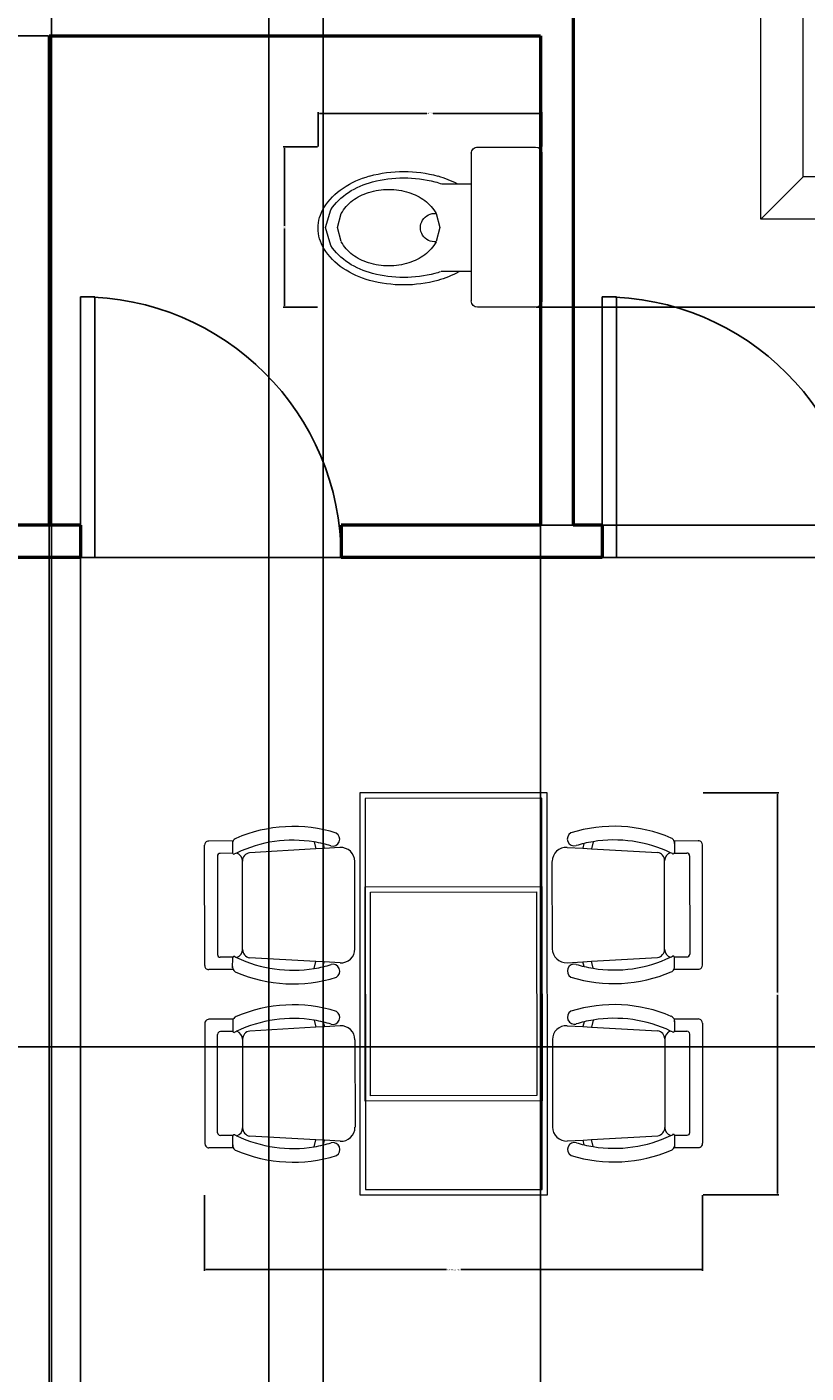
# Model space of a CAD drawing. Units: inches. Extents: x -108 to 1456, y -102 to 617.
# Tile 5 of 8: x 345 to 453, y 337 to 523. Entities that reach past the tile are written whole.
import ezdxf

# ---------------------------------------------------------------- set-up
doc = ezdxf.new("R2010")
doc.units = ezdxf.units.IN
for name, color, linetype, lineweight in [('A-ANNO-DIMS', 2, 'Continuous', 18), ('A-DOOR', 3, 'Continuous', 25), ('A-FLOR-FIXT', 9, 'Continuous', 20), ('A-FURN', 8, 'Continuous', 18), ('A-WALL', 7, 'Continuous', 50)]:
    doc.layers.add(name, color=color, linetype=linetype, lineweight=lineweight)
doc.styles.get("Standard").update_dxf_attribs({"font": 'arial.ttf'})
doc.dimstyles.get("Standard").update_dxf_attribs({"dimtxt": 0.18, "dimasz": 0.18, "dimexe": 0.18, "dimexo": 0.0625, "dimgap": 0.09, "dimtad": 0, "dimtih": 1, "dimtoh": 1, "dimdec": 4, "dimzin": 0, "dimdsep": 46, "dimtxsty": 'Standard', "dimcen": 0.09, "dimadec": 0, "dimazin": 0, "dimtfac": 1, "dimtdec": 4, "dimtofl": 0, "dimtmove": 0, "dimatfit": 3, "dimfxl": 1, "dimtolj": 1, "dimtzin": 0, "dimarcsym": 0})

# ---------------------------------------------------------------- blocks, each defined once
blk = doc.blocks.new('A$C50B66110')
for p, q in [((0.0153, 1.9631), (0.0153, 1.5831)), ((0.0503, 1.9981), (0.4803, 1.9981)), ((0.1513, 1.6871), (0.1513, 1.9967)), ((0.5153, 1.9631), (0.5153, 1.5831)), ((0.5716, 1.9488), (0.5716, 2)), ((0.5716, 2), (2.0719, 2)), ((2.0719, 1.9488), (2.0719, 2)), ((2.1051, 1.9643), (2.1051, 1.5843)), ((2.5701, 1.9993), (2.1401, 1.9993)), ((2.6051, 1.9643), (2.6051, 1.5843)), ((0.0653, 1.9481), (0.0653, 1.5981)), ((0.0653, 1.9481), (0.4653, 1.9481)), ((0.4653, 1.9481), (0.4653, 1.5981)), ((2.0719, 1.9488), (0.5716, 1.9488)), ((0.5716, 1.9488), (0.5716, 0)), ((2.0719, 0), (2.0719, 1.9488)), ((2.1551, 1.9493), (2.1551, 1.5993)), ((2.5551, 1.9493), (2.1551, 1.9493)), ((2.3505, 1.62), (2.3505, 1.9295)), ((2.5551, 1.9493), (2.5551, 1.5993)), ((0.7257, 1.5725), (0.7257, 1.8954)), ((0.7257, 1.8954), (1.2113, 1.8954)), ((1.2113, 1.8954), (1.2113, 1.5725)), ((1.4007, 1.5725), (1.4007, 1.8954)), ((1.4007, 1.8954), (1.8863, 1.8954)), ((1.8863, 1.8954), (1.8863, 1.5725)), ((0, 1.8416), (0.2001, 1.8416)), ((2.5018, 1.7744), (2.2017, 1.7744)), ((0.0653, 1.5981), (0.4653, 1.5981)), ((2.5551, 1.5993), (2.1551, 1.5993)), ((0.0503, 1.5481), (0.4803, 1.5481)), ((1.2113, 1.5725), (0.7257, 1.5725)), ((1.8863, 1.5725), (1.4007, 1.5725)), ((2.5701, 1.5493), (2.1401, 1.5493)), ((1.5665, 1.5254), (1.5665, 1.0802)), ((1.5665, 1.5254), (1.9219, 1.0802)), ((1.9219, 1.0802), (1.5665, 1.0802)), ((0.5716, 0), (0.7216, 0.15)), ((2.0719, 0), (1.9219, 0.15)), ((0.5716, 0), (2.0719, 0))]:
    blk.add_line(p, q)
at = {"linetype": 'ByBlock'}
for p, q in [((0.2481, 1.9162), (0.2458, 1.9139)), ((0.2458, 1.9139), (0.2458, 1.7562)), ((0.2481, 1.9162), (0.4287, 1.9162)), ((0.3772, 1.9071), (0.3818, 1.9128)), ((0.3818, 1.9094), (0.3807, 1.9048)), ((0.3818, 1.9128), (0.4161, 1.9128)), ((0.3864, 1.9116), (0.3818, 1.9094)), ((0.3921, 1.8968), (0.3864, 1.9116)), ((0.3864, 1.9116), (0.4138, 1.9116)), ((0.4081, 1.8968), (0.4138, 1.9116)), ((0.4138, 1.9116), (0.4184, 1.9094)), ((0.4161, 1.9128), (0.4218, 1.9071)), ((0.4184, 1.9094), (0.4195, 1.9048)), ((0.4287, 1.9162), (0.4309, 1.9139)), ((0.4309, 1.9139), (0.4309, 1.7562)), ((0.2526, 1.9036), (0.2526, 1.8431)), ((0.3669, 1.9036), (0.2526, 1.9036)), ((0.3669, 1.8431), (0.3669, 1.9036)), ((0.3772, 1.7688), (0.3772, 1.9071)), ((0.3807, 1.9048), (0.3807, 1.8739)), ((0.3807, 1.9048), (0.3909, 1.8945)), ((0.3807, 1.8739), (0.3829, 1.8682)), ((0.3829, 1.8682), (0.3864, 1.8625)), ((0.3864, 1.8625), (0.3875, 1.8545)), ((0.3909, 1.8945), (0.3921, 1.8968)), ((0.3909, 1.8431), (0.3909, 1.8945)), ((0.4081, 1.8968), (0.3921, 1.8968)), ((0.4092, 1.8945), (0.4081, 1.8968)), ((0.4195, 1.9048), (0.4092, 1.8945)), ((0.4092, 1.8431), (0.4092, 1.8945)), ((0.4138, 1.8625), (0.4127, 1.8545)), ((0.4172, 1.8682), (0.4138, 1.8625)), ((0.4195, 1.8739), (0.4172, 1.8682)), ((0.4195, 1.9048), (0.4195, 1.8739)), ((0.4218, 1.9071), (0.4218, 1.7699)), ((0.2526, 1.8431), (0.3669, 1.8431)), ((0.3201, 1.8168), (0.2526, 1.8168)), ((0.2526, 1.8168), (0.2526, 1.7962)), ((0.2572, 1.8408), (0.2572, 1.8294)), ((0.3669, 1.8408), (0.2572, 1.8408)), ((0.2572, 1.8294), (0.3669, 1.8294)), ((0.2675, 1.8145), (0.2641, 1.8145)), ((0.2641, 1.8145), (0.2641, 1.8111)), ((0.2664, 1.8408), (0.2664, 1.8294)), ((0.2675, 1.8111), (0.2675, 1.8145)), ((0.2755, 1.8408), (0.2755, 1.8294)), ((0.2846, 1.8408), (0.2846, 1.8294)), ((0.2846, 1.8145), (0.2846, 1.8111)), ((0.2881, 1.8145), (0.2846, 1.8145)), ((0.2881, 1.8111), (0.2881, 1.8145)), ((0.2938, 1.8408), (0.2938, 1.8294)), ((0.3029, 1.8408), (0.3029, 1.8294)), ((0.3052, 1.8145), (0.3052, 1.8111)), ((0.3086, 1.8145), (0.3052, 1.8145)), ((0.3086, 1.8111), (0.3086, 1.8145)), ((0.3121, 1.8408), (0.3121, 1.8294)), ((0.3201, 1.7962), (0.3201, 1.8168)), ((0.3669, 1.8294), (0.3669, 1.8408)), ((0.3829, 1.8076), (0.3864, 1.8134)), ((0.3864, 1.8134), (0.3875, 1.8214)), ((0.3875, 1.8545), (0.3875, 1.8431)), ((0.3875, 1.8214), (0.3875, 1.8431)), ((0.3909, 1.8431), (0.3909, 1.7813)), ((0.4092, 1.8431), (0.4092, 1.7813)), ((0.4127, 1.8545), (0.4127, 1.8431)), ((0.4127, 1.8214), (0.4127, 1.8431)), ((0.4138, 1.8134), (0.4127, 1.8214)), ((0.4172, 1.8076), (0.4138, 1.8134)), ((0.2526, 1.7962), (0.3201, 1.7962)), ((0.2652, 1.7905), (0.2538, 1.7905)), ((0.2538, 1.7905), (0.2538, 1.7859)), ((0.2538, 1.7859), (0.2652, 1.7859)), ((0.2538, 1.7665), (0.2538, 1.7733)), ((0.2538, 1.7733), (0.2652, 1.7733)), ((0.2652, 1.7665), (0.2538, 1.7665)), ((0.2641, 1.8111), (0.2675, 1.8111)), ((0.2641, 1.8019), (0.2641, 1.7985)), ((0.2675, 1.8019), (0.2641, 1.8019)), ((0.2641, 1.7985), (0.2675, 1.7985)), ((0.2652, 1.7859), (0.2652, 1.7905)), ((0.2652, 1.7733), (0.2652, 1.7665)), ((0.2675, 1.7985), (0.2675, 1.8019)), ((0.2812, 1.7905), (0.2698, 1.7905)), ((0.2698, 1.7905), (0.2698, 1.7859)), ((0.2698, 1.7859), (0.2812, 1.7859)), ((0.2698, 1.7665), (0.2698, 1.7733)), ((0.2698, 1.7733), (0.2812, 1.7733)), ((0.2812, 1.7665), (0.2698, 1.7665)), ((0.2812, 1.7859), (0.2812, 1.7905)), ((0.2812, 1.7733), (0.2812, 1.7665)), ((0.2846, 1.8111), (0.2881, 1.8111)), ((0.2846, 1.8019), (0.2846, 1.7985)), ((0.2881, 1.8019), (0.2846, 1.8019)), ((0.2846, 1.7985), (0.2881, 1.7985)), ((0.2972, 1.7905), (0.2858, 1.7905)), ((0.2858, 1.7905), (0.2858, 1.7859)), ((0.2858, 1.7859), (0.2972, 1.7859)), ((0.2858, 1.7665), (0.2858, 1.7733)), ((0.2858, 1.7733), (0.2972, 1.7733)), ((0.2972, 1.7665), (0.2858, 1.7665)), ((0.2881, 1.7985), (0.2881, 1.8019)), ((0.2972, 1.7859), (0.2972, 1.7905)), ((0.2972, 1.7733), (0.2972, 1.7665)), ((0.3018, 1.7905), (0.3018, 1.7859)), ((0.3132, 1.7905), (0.3018, 1.7905)), ((0.3018, 1.7859), (0.3132, 1.7859)), ((0.3018, 1.7733), (0.3132, 1.7733)), ((0.3018, 1.7665), (0.3018, 1.7733)), ((0.3132, 1.7665), (0.3018, 1.7665)), ((0.3052, 1.8111), (0.3086, 1.8111)), ((0.3052, 1.8019), (0.3052, 1.7985)), ((0.3086, 1.8019), (0.3052, 1.8019)), ((0.3052, 1.7985), (0.3086, 1.7985)), ((0.3086, 1.7985), (0.3086, 1.8019)), ((0.3132, 1.7859), (0.3132, 1.7905)), ((0.3132, 1.7733), (0.3132, 1.7665)), ((0.3304, 1.8111), (0.3395, 1.8111)), ((0.3304, 1.8042), (0.3304, 1.8111)), ((0.3395, 1.8042), (0.3304, 1.8042)), ((0.3304, 1.7985), (0.3395, 1.7985)), ((0.3304, 1.7916), (0.3304, 1.7985)), ((0.3395, 1.7916), (0.3304, 1.7916)), ((0.3304, 1.7779), (0.3304, 1.7848)), ((0.3304, 1.7848), (0.3395, 1.7848)), ((0.3395, 1.7779), (0.3304, 1.7779)), ((0.3304, 1.7722), (0.3395, 1.7722)), ((0.3304, 1.7653), (0.3304, 1.7722)), ((0.3395, 1.8111), (0.3395, 1.8042)), ((0.3395, 1.7985), (0.3395, 1.7916)), ((0.3395, 1.7848), (0.3395, 1.7779)), ((0.3395, 1.7722), (0.3395, 1.7653)), ((0.3441, 1.8042), (0.3441, 1.8111)), ((0.3441, 1.8111), (0.3532, 1.8111)), ((0.3532, 1.8042), (0.3441, 1.8042)), ((0.3441, 1.7985), (0.3532, 1.7985)), ((0.3441, 1.7916), (0.3441, 1.7985)), ((0.3532, 1.7916), (0.3441, 1.7916)), ((0.3441, 1.7779), (0.3441, 1.7848)), ((0.3441, 1.7848), (0.3532, 1.7848)), ((0.3532, 1.7779), (0.3441, 1.7779)), ((0.3441, 1.7722), (0.3532, 1.7722)), ((0.3441, 1.7653), (0.3441, 1.7722)), ((0.3532, 1.8111), (0.3532, 1.8042)), ((0.3532, 1.7985), (0.3532, 1.7916)), ((0.3532, 1.7848), (0.3532, 1.7779)), ((0.3532, 1.7722), (0.3532, 1.7653)), ((0.3578, 1.8111), (0.3669, 1.8111)), ((0.3578, 1.8042), (0.3578, 1.8111)), ((0.3669, 1.8042), (0.3578, 1.8042)), ((0.3578, 1.7985), (0.3669, 1.7985)), ((0.3578, 1.7916), (0.3578, 1.7985)), ((0.3669, 1.7916), (0.3578, 1.7916)), ((0.3578, 1.7791), (0.3578, 1.7859)), ((0.3578, 1.7859), (0.3669, 1.7859)), ((0.3669, 1.7791), (0.3578, 1.7791)), ((0.3578, 1.7653), (0.3578, 1.7722)), ((0.3578, 1.7722), (0.3669, 1.7722)), ((0.3669, 1.8111), (0.3669, 1.8042)), ((0.3669, 1.7985), (0.3669, 1.7916)), ((0.3669, 1.7859), (0.3669, 1.7791)), ((0.3669, 1.7722), (0.3669, 1.7653)), ((0.3829, 1.7631), (0.3772, 1.7688)), ((0.3807, 1.8019), (0.3829, 1.8076)), ((0.3807, 1.7711), (0.3807, 1.8019)), ((0.3807, 1.7711), (0.3909, 1.7813)), ((0.3818, 1.7665), (0.3807, 1.7711)), ((0.3864, 1.7642), (0.3818, 1.7665)), ((0.3921, 1.7791), (0.3864, 1.7642)), ((0.3909, 1.7813), (0.3921, 1.7791)), ((0.4081, 1.7791), (0.3921, 1.7791)), ((0.4024, 1.7676), (0.3989, 1.7676)), ((0.3989, 1.7676), (0.3991, 1.7578)), ((0.403, 1.7585), (0.4024, 1.7676)), ((0.4092, 1.7813), (0.4081, 1.7791)), ((0.4081, 1.7791), (0.4138, 1.7642)), ((0.4195, 1.7711), (0.4092, 1.7813)), ((0.4138, 1.7642), (0.4184, 1.7665)), ((0.4218, 1.7699), (0.4161, 1.7631)), ((0.4195, 1.8019), (0.4172, 1.8076)), ((0.4184, 1.7665), (0.4195, 1.7711)), ((0.4195, 1.7711), (0.4195, 1.8019)), ((0.4378, 1.7742), (0.4309, 1.7768)), ((0.4309, 1.7722), (0.436, 1.7708)), ((0.436, 1.7708), (0.4406, 1.7672)), ((0.441, 1.771), (0.4378, 1.7742)), ((0.4406, 1.7672), (0.4418, 1.7656)), ((0.4434, 1.7688), (0.441, 1.771)), ((0.4443, 1.7658), (0.4418, 1.7633)), ((0.4418, 1.7656), (0.4443, 1.7658)), ((0.4477, 1.7704), (0.4434, 1.7688)), ((0.4497, 1.7684), (0.4477, 1.7704)), ((0.4481, 1.765), (0.4497, 1.7684)), ((0.4509, 1.7672), (0.4481, 1.765)), ((0.4539, 1.764), (0.4509, 1.7672)), ((0.2458, 1.7562), (0.2481, 1.7539)), ((0.4, 1.7539), (0.2481, 1.7539)), ((0.3395, 1.7653), (0.3304, 1.7653)), ((0.3532, 1.7653), (0.3441, 1.7653)), ((0.3669, 1.7653), (0.3578, 1.7653)), ((0.399, 1.7631), (0.3829, 1.7631)), ((0.3864, 1.7642), (0.399, 1.7642)), ((0.3991, 1.7578), (0.4019, 1.7462)), ((0.4019, 1.7462), (0.4047, 1.7353)), ((0.4026, 1.7254), (0.4021, 1.7198)), ((0.4021, 1.7198), (0.4088, 1.7187)), ((0.4088, 1.7187), (0.4023, 1.7147)), ((0.4026, 1.7642), (0.4138, 1.7642)), ((0.4051, 1.7279), (0.4026, 1.7254)), ((0.4161, 1.7631), (0.4027, 1.7631)), ((0.4047, 1.7511), (0.403, 1.7585)), ((0.4287, 1.7539), (0.404, 1.7539)), ((0.4047, 1.7353), (0.4044, 1.7293)), ((0.4044, 1.7293), (0.4051, 1.7279)), ((0.4074, 1.7402), (0.4047, 1.7511)), ((0.4081, 1.7346), (0.4074, 1.7402)), ((0.4079, 1.7286), (0.4081, 1.7346)), ((0.4121, 1.7256), (0.4079, 1.7286)), ((0.4111, 1.7203), (0.4121, 1.7256)), ((0.4123, 1.7057), (0.4111, 1.7203)), ((0.4309, 1.7562), (0.4287, 1.7539)), ((0.4418, 1.7633), (0.4511, 1.7551)), ((0.4511, 1.7551), (0.4662, 1.7422)), ((0.4515, 1.7573), (0.4539, 1.764)), ((0.4577, 1.7605), (0.4515, 1.7573)), ((0.463, 1.7555), (0.4577, 1.7605)), ((0.4618, 1.7482), (0.463, 1.7555)), ((0.467, 1.7515), (0.4618, 1.7482)), ((0.4664, 1.7418), (0.4741, 1.72)), ((0.4714, 1.7468), (0.467, 1.7515)), ((0.4696, 1.7418), (0.4714, 1.7468)), ((0.4766, 1.7425), (0.4697, 1.7418)), ((0.4741, 1.72), (0.4708, 1.7027)), ((0.472, 1.733), (0.4787, 1.7356)), ((0.4794, 1.7332), (0.472, 1.733)), ((0.4761, 1.7233), (0.481, 1.7279)), ((0.4824, 1.7233), (0.4761, 1.7233)), ((0.4787, 1.7356), (0.4766, 1.7425)), ((0.481, 1.7279), (0.4794, 1.7332)), ((0.4835, 1.7175), (0.4824, 1.7233)), ((0.4023, 1.7147), (0.4028, 1.7085)), ((0.4028, 1.7085), (0.4102, 1.7078)), ((0.4102, 1.7078), (0.4037, 1.7027)), ((0.4037, 1.7027), (0.4067, 1.6974)), ((0.4067, 1.6974), (0.4137, 1.6988)), ((0.4137, 1.6988), (0.4104, 1.6923)), ((0.4104, 1.6923), (0.4139, 1.6881)), ((0.4211, 1.6946), (0.4123, 1.7057)), ((0.4139, 1.6881), (0.4192, 1.692)), ((0.4192, 1.692), (0.4183, 1.6858)), ((0.4183, 1.6858), (0.4227, 1.683)), ((0.4333, 1.6881), (0.4211, 1.6946)), ((0.4227, 1.683), (0.4283, 1.6876)), ((0.4283, 1.6876), (0.4276, 1.68)), ((0.4276, 1.68), (0.4324, 1.6786)), ((0.4324, 1.6786), (0.4354, 1.6849)), ((0.4472, 1.6869), (0.4333, 1.6881)), ((0.4354, 1.6849), (0.4382, 1.6786)), ((0.4382, 1.6786), (0.4421, 1.6782)), ((0.4421, 1.6782), (0.4437, 1.6849)), ((0.4437, 1.6849), (0.4463, 1.6775)), ((0.4463, 1.6775), (0.4507, 1.6786)), ((0.4606, 1.6927), (0.4472, 1.6869)), ((0.4507, 1.6786), (0.4509, 1.6849)), ((0.4509, 1.6849), (0.4562, 1.6802)), ((0.4562, 1.6802), (0.4599, 1.6821)), ((0.4592, 1.689), (0.4641, 1.683)), ((0.4599, 1.6821), (0.4592, 1.689)), ((0.4708, 1.7027), (0.4606, 1.6927)), ((0.4641, 1.683), (0.4678, 1.6863)), ((0.465, 1.6925), (0.4715, 1.6897)), ((0.4678, 1.6863), (0.465, 1.6925)), ((0.4745, 1.6925), (0.4713, 1.6988)), ((0.4713, 1.6988), (0.478, 1.6967)), ((0.4715, 1.6897), (0.4745, 1.6925)), ((0.4743, 1.7075), (0.4815, 1.7073)), ((0.4798, 1.7013), (0.4743, 1.7075)), ((0.4764, 1.7154), (0.4835, 1.7175)), ((0.4824, 1.7119), (0.4764, 1.7154)), ((0.478, 1.6967), (0.4798, 1.7013)), ((0.4815, 1.7073), (0.4824, 1.7119)), ((0.7216, 1.5254), (1.9219, 1.5254)), ((0.7216, 1.5254), (0.7216, 0.15)), ((1.9219, 0.15), (1.9219, 1.5254)), ((0.7216, 0.15), (1.9219, 0.15))]:
    blk.add_line(p, q, dxfattribs=at)
for centre, radius in [((0.1513, 1.8416), 0.12), ((0.1513, 1.8416), 0.06), ((2.3505, 1.7744), 0.12), ((2.3505, 1.7744), 0.06)]:
    blk.add_circle(centre, radius)
for centre, radius, start, end in [((0.0153, 1.9981), 0.035, 270, 0), ((0.5153, 1.9981), 0.035, 180, 270), ((2.1051, 1.9993), 0.035, 270, 0), ((2.6051, 1.9993), 0.035, 180, 270), ((0.6244, 1.734), 0.1906, 302.1202, 57.8798), ((1.3126, 1.734), 0.1906, 122.1202, 237.8798), ((1.2994, 1.734), 0.1906, 302.1202, 57.8798), ((1.9876, 1.734), 0.1906, 122.1202, 237.8798), ((0.0153, 1.5481), 0.035, 0, 90), ((0.5153, 1.5481), 0.035, 90, 180), ((2.1051, 1.5493), 0.035, 0, 90), ((2.6051, 1.5493), 0.035, 90, 180), ((1.1502, 0.7366), 0.3575, 102.4782, 140.4625), ((0.328, 0.4368), 0.9879, 28.4971, 41.0566), ((1.9117, 1.3157), 0.8697, 195.336, 226.4193), ((0.9996, 0.4307), 0.548, 103.2034, 117.0362), ((1.656, 1.7093), 1.0798, 223.6306, 251.4288), ((0.4482, 0.4408), 0.5655, 5.3391, 57.6895), ((1.8226, 1.3753), 1.1652, 203.0642, 220.3209), ((0.4548, 0.5307), 0.4879, 10.6986, 52.6864), ((0.5648, 0.4378), 0.7874, 18.3527, 36.6851), ((-0.0179, 2.4352), 2.1977, 305.2966, 307.2418), ((1.5981, 0.9345), 0.734, 205.259, 216.9351), ((1.4166, 0.4903), 0.3575, 154.0418, 192.0262), ((1.1403, -0.3401), 0.9879, 80.0607, 92.6202), ((1.2867, -0.154), 0.7874, 69.9163, 88.2487), ((1.3672, 0.0075), 0.6085, 71.81, 120.1351), ((1.4431, 0.1219), 0.4774, 76.1849, 142.0017), ((-0.6401, 0.6314), 2.1977, 349.4884, 358.8054), ((-0.0179, 2.4352), 2.1977, 297.9248, 299.3793), ((1.5626, 0.1822), 0.548, 154.767, 168.5998), ((1.3343, 1.4141), 1.1652, 254.6278, 271.8845), ((1.2678, 0.9611), 0.6885, 250.2936, 293.6414), ((1.5399, 0.9642), 0.734, 256.8226, 268.4988)]:
    blk.add_arc(centre, radius, start, end)
blk = doc.blocks.new('A$C7D96336B')
for p, q in [((280, 0.2), (-280, -0.2)), ((280.8, -1199.8), (280, 0.2)), ((-280, -0.2), (-279.2, -1200.2)), ((264, -15.8), (-264, -16.2)), ((-264, -16.2), (-263.2, -1184.2)), ((264.8, -1183.8), (264, -15.8)), ((-742.8, -515.1), (-743.2, -156.2)), ((-658.1, -143.4), (-730.7, -143.6)), ((-659.8, -143.4), (-659.7, -178.7)), ((-416.5, -146.3), (-411.5, -167.3)), ((-389.5, -151.7), (-386.1, -165.8)), ((389.7, -151.1), (386.3, -165.3)), ((416.7, -145.7), (411.7, -166.7)), ((658.3, -142.5), (730.9, -142.6)), ((659.9, -142.6), (659.9, -177.8)), ((743.5, -514.1), (743.4, -155.2)), ((-704.9, -188.8), (-704.6, -482.3)), ((-659.3, -180.3), (-696.6, -180.5)), ((-411.5, -167.3), (-609.1, -178.7)), ((-386.1, -165.8), (-411.5, -167.3)), ((-338.9, -163.1), (-386.1, -165.8)), ((339.1, -162.6), (386.3, -165.3)), ((386.3, -165.3), (411.7, -166.7)), ((411.7, -166.7), (609.3, -177.8)), ((659.5, -179.5), (696.9, -179.5)), ((705.2, -187.9), (705.3, -481.4)), ((-629.9, -467.6), (-630.2, -203.4)), ((-294.5, -465.7), (-294.4, -204.7)), ((295.2, -465.3), (294.7, -204.3)), ((630.5, -466.8), (630.5, -202.5)), ((-263.8, -280.2), (264.2, -279.8)), ((-263.8, -280.2), (264.2, -279.8)), ((-263.4, -920.2), (-263.8, -280.2)), ((264.2, -279.8), (264.6, -919.8)), ((-247.8, -296.2), (248.2, -295.8)), ((-247.4, -904.2), (-247.8, -296.2)), ((248.2, -295.8), (248.6, -903.8)), ((-659, -490.7), (-696.3, -490.7)), ((-659.4, -522.3), (-659.3, -492.4)), ((-411.1, -503.3), (-608.7, -492.3)), ((-416.1, -524.3), (-411.1, -503.3)), ((-385.8, -504.7), (-411.1, -503.3)), ((-389.1, -518.8), (-385.8, -504.7)), ((-338.5, -507.3), (-385.8, -504.7)), ((339.2, -506.9), (386.5, -504.2)), ((386.5, -504.2), (411.8, -502.7)), ((389.8, -518.3), (386.5, -504.2)), ((411.8, -502.7), (609.4, -491.4)), ((416.8, -523.7), (411.8, -502.7)), ((659.6, -489.8), (697, -489.7)), ((660.1, -521.4), (660, -491.5)), ((-657.7, -527.6), (-730.3, -527.6)), ((658.4, -526.7), (731, -526.6)), ((-657.6, -675.8), (-730.2, -675.9)), ((-659.3, -681), (-659.2, -711)), ((-416, -678.8), (-411, -699.8)), ((416.9, -678.2), (411.9, -699.2)), ((658.5, -674.9), (731.1, -674.9)), ((660.2, -680.2), (660.2, -710.1)), ((-742.7, -688.4), (-742.6, -1047.3)), ((-704.4, -1014.6), (-704.5, -721.1)), ((-658.8, -712.7), (-696.2, -712.8)), ((-411, -699.8), (-608.6, -711)), ((-385.6, -698.3), (-411, -699.8)), ((-389, -684.2), (-385.6, -698.3)), ((-338.4, -695.6), (-385.6, -698.3)), ((339.3, -695.2), (386.6, -697.8)), ((389.9, -683.7), (386.6, -697.8)), ((386.6, -697.8), (411.9, -699.2)), ((411.9, -699.2), (609.5, -710.2)), ((659.8, -711.8), (697.1, -711.8)), ((705.8, -1013.7), (705.5, -720.2)), ((743.6, -687.4), (744, -1046.3)), ((-629.7, -735.7), (-629.6, -1000)), ((-294.4, -737.1), (-293.9, -998.2)), ((295.3, -736.7), (295.2, -997.8)), ((630.7, -734.9), (631, -999.1)), ((264.6, -919.8), (-263.4, -920.2)), ((248.6, -903.8), (-247.4, -904.2)), ((-658.7, -1023), (-696.1, -1023)), ((-659.1, -1059.9), (-659.1, -1024.7)), ((-410.9, -1035.8), (-608.5, -1024.6)), ((-415.9, -1056.8), (-410.9, -1035.8)), ((-385.5, -1037.2), (-410.9, -1035.8)), ((-388.9, -1051.4), (-385.5, -1037.2)), ((-338.3, -1039.9), (-385.5, -1037.2)), ((339.7, -1039.4), (386.9, -1036.7)), ((386.9, -1036.7), (412.3, -1035.2)), ((390.3, -1050.8), (386.9, -1036.7)), ((412.3, -1035.2), (609.9, -1023.8)), ((417.3, -1056.2), (412.3, -1035.2)), ((660.1, -1022.1), (697.4, -1022)), ((660.6, -1059), (660.5, -1023.8)), ((-657.5, -1059.9), (-730.1, -1059.9)), ((658.9, -1059), (731.5, -1058.9)), ((-279.2, -1200.2), (280.8, -1199.8)), ((-263.2, -1184.2), (264.8, -1183.8))]:
    blk.add_line(p, q)
for centre, radius, start, end in [((-478.6, -532.7), 432.3, 72.7119, 113.3258), ((-360.6, -137.9), 20.8, 254.7795, 60.0186), ((360.7, -137.4), 20.8, 120.0589, 285.298), ((479.4, -532), 432.3, 66.7517, 107.3656), ((-730.7, -156.1), 12.5, 141.7605, 180.1459), ((-730.7, -156.1), 12.5, 90.1463, 141.7605), ((-643.2, -151), 16.7, 153.004, 184.8567), ((-643.2, -151), 16.7, 113.3258, 153.004), ((-479.1, -531.9), 390.7, 80.7703, 115.5809), ((-479.1, -531.9), 390.7, 76.7336, 80.7703), ((-479.1, -531.9), 390.7, 73.1676, 76.7336), ((479.9, -531.2), 390.7, 103.3439, 106.9099), ((479.9, -531.2), 390.7, 99.3072, 103.3439), ((479.9, -531.2), 390.7, 64.4966, 99.3072), ((643.4, -150.1), 16.7, 27.0735, 66.7517), ((643.4, -150.1), 16.7, 355.2209, 27.0735), ((730.9, -155.1), 12.5, 38.317, 89.9312), ((730.9, -155.1), 12.5, 359.9316, 38.317), ((-696.6, -188.8), 8.33, 90.1463, 180.1463), ((-655.5, -178.6), 4.17, 180.1463, 296.5296), ((-479.1, -531.9), 390.7, 115.5809, 116.5296), ((-655.2, -203.4), 25, 0.1463, 72.8968), ((-605.2, -203.4), 25, 98.9209, 179.9714), ((-336.5, -204.7), 41.7, 0.1463, 93.3068), ((336.7, -204.2), 41.7, 86.7707, 179.9312), ((605.5, -202.6), 25, 0.1061, 81.1566), ((655.5, -202.5), 25, 107.1807, 179.9312), ((479.9, -531.2), 390.7, 63.5479, 64.4966), ((655.7, -177.8), 4.17, 243.5479, 359.9312), ((696.9, -187.8), 8.33, 359.9312, 89.9312), ((-696.3, -482.3), 8.33, 179.9714, 269.9714), ((-654.9, -467.6), 25, 287.2209, 359.9714), ((-604.9, -467.6), 25, 180.1463, 261.1967), ((-336.2, -465.7), 41.7, 266.8108, 359.9714), ((336.8, -465.3), 41.7, 180.1061, 273.2667), ((605.5, -466.7), 25, 278.8808, 359.9312), ((655.5, -466.7), 25, 180.1061, 252.8566), ((697, -481.4), 8.33, 270.1061, 0.1061), ((-730.3, -515.1), 12.5, 179.9717, 218.3572), ((-642.9, -520), 16.7, 175.261, 207.1136), ((-655.2, -492.4), 4.17, 63.5881, 179.9714), ((-479.5, -138.8), 390.7, 243.5881, 244.5368), ((-479.5, -138.8), 390.7, 244.5368, 279.3474), ((-479.5, -138.8), 390.7, 279.3474, 283.3841), ((-479.5, -138.8), 390.7, 283.3841, 286.9501), ((-360.2, -532.5), 20.8, 300.0991, 105.3382), ((360.9, -532), 20.8, 74.7393, 239.9785), ((479.7, -138.1), 390.7, 253.1274, 256.6934), ((479.7, -138.1), 390.7, 256.6934, 260.7301), ((479.7, -138.1), 390.7, 260.7301, 295.5407), ((479.7, -138.1), 390.7, 295.5407, 296.4894), ((655.8, -491.5), 4.17, 0.1061, 116.4894), ((643.6, -519.1), 16.7, 332.9639, 4.8165), ((731, -514.1), 12.5, 270.1061, 321.7203), ((731, -514.1), 12.5, 321.7203, 0.1058), ((-730.3, -515.1), 12.5, 218.3572, 269.9714), ((-642.9, -520), 16.7, 207.1136, 246.7919), ((-479.1, -138), 432.3, 246.7919, 287.4058), ((479.2, -137.3), 432.3, 252.6717, 293.2857), ((643.6, -519.1), 16.7, 293.2857, 332.9639), ((-478.4, -1065.1), 432.3, 72.6717, 113.2857), ((479.9, -1064.5), 432.3, 66.7919, 107.4058), ((-730.2, -688.4), 12.5, 141.7203, 180.1058), ((-730.2, -688.4), 12.5, 90.1061, 141.7203), ((-642.7, -683.3), 16.7, 152.9639, 184.8165), ((-642.7, -683.3), 16.7, 113.2857, 152.9639), ((-478.9, -1064.3), 390.7, 80.7301, 115.5407), ((-478.9, -1064.3), 390.7, 76.6934, 80.7301), ((-360.1, -670.4), 20.8, 254.7393, 59.9785), ((361, -670), 20.8, 120.0991, 285.3382), ((480.4, -1063.7), 390.7, 99.3474, 103.3841), ((480.4, -1063.7), 390.7, 64.5368, 99.3474), ((643.7, -682.5), 16.7, 27.1136, 66.7919), ((643.7, -682.5), 16.7, 355.261, 27.1136), ((731.1, -687.4), 12.5, 38.3572, 89.9714), ((731.1, -687.4), 12.5, 359.9717, 38.3572), ((-696.1, -721.1), 8.33, 90.1061, 180.1061), ((-655, -711), 4.17, 180.1061, 296.4894), ((-478.9, -1064.3), 390.7, 115.5407, 116.4894), ((-654.7, -735.8), 25, 0.1061, 72.8566), ((-604.7, -735.7), 25, 98.8808, 179.9312), ((-478.9, -1064.3), 390.7, 73.1274, 76.6934), ((-336, -737.2), 41.7, 0.1061, 93.2667), ((337, -736.8), 41.7, 86.8108, 179.9714), ((480.4, -1063.7), 390.7, 103.3841, 106.9501), ((605.7, -734.9), 25, 0.1463, 81.1967), ((655.7, -734.9), 25, 107.2209, 179.9714), ((480.4, -1063.7), 390.7, 63.5881, 64.5368), ((656, -710.1), 4.17, 243.5881, 359.9714), ((697.1, -720.1), 8.33, 359.9714, 89.9714), ((-654.6, -1000), 25, 287.1807, 359.9312), ((-604.6, -999.9), 25, 180.1061, 261.1566), ((-335.9, -998.3), 41.7, 266.7707, 359.9312), ((337.3, -997.8), 41.7, 180.1463, 273.3068), ((606, -999.1), 25, 278.9209, 359.9714), ((656, -999.1), 25, 180.1463, 252.8968), ((-696.1, -1014.6), 8.33, 179.9312, 269.9312), ((-654.9, -1024.7), 4.17, 63.5479, 179.9312), ((-479.1, -671.2), 390.7, 243.5479, 244.4966), ((-479.1, -671.2), 390.7, 244.4966, 279.3072), ((-479.1, -671.2), 390.7, 283.3439, 286.9099), ((-359.9, -1065.1), 20.8, 300.0589, 105.298), ((361.4, -1064.6), 20.8, 74.7795, 240.0186), ((480, -670.6), 390.7, 253.1676, 256.7336), ((480, -670.6), 390.7, 260.7703, 295.5809), ((480, -670.6), 390.7, 295.5809, 296.5296), ((656.3, -1023.8), 4.17, 0.1463, 116.5296), ((697.4, -1013.7), 8.33, 270.1463, 0.1463), ((-730.1, -1047.4), 12.5, 179.9316, 218.317), ((-730.1, -1047.4), 12.5, 218.317, 269.9312), ((-642.6, -1052.4), 16.7, 175.2209, 207.0735), ((-642.6, -1052.4), 16.7, 207.0735, 246.7517), ((-478.6, -670.4), 432.3, 246.7517, 287.3656), ((-479.1, -671.2), 390.7, 279.3072, 283.3439), ((479.5, -669.8), 432.3, 252.7119, 293.3258), ((480, -670.6), 390.7, 256.7336, 260.7703), ((644, -1051.5), 16.7, 293.3258, 333.004), ((644, -1051.5), 16.7, 333.004, 4.8567), ((731.5, -1046.4), 12.5, 270.1463, 321.7605), ((731.5, -1046.4), 12.5, 321.7605, 0.1459)]:
    blk.add_arc(centre, radius, start, end)
blk = doc.blocks.new('A$C44022395')
for p, q in [((0, 0.6877), (0, 0.5044)), ((0.4866, 0.7077), (0.02, 0.7077)), ((0.5066, 0.5044), (0.5066, 0.6877)), ((0.4866, 0.4844), (0.02, 0.4844)), ((0.1134, 0.4844), (0.1134, 0.389)), ((0.3892, 0.4844), (0.3892, 0.3908)), ((0.2517, 0.3846), (0.2074, 0.3731)), ((0.2959, 0.3731), (0.2517, 0.3846)), ((0.2074, 0.0734), (0.2517, 0.0619)), ((0.2517, 0.0619), (0.2959, 0.0734)), ((0.1955, 0.0404), (0.2517, 0.0238)), ((0.2517, 0.0238), (0.3078, 0.0404))]:
    blk.add_line(p, q)
for centre, radius, start, end in [((0.02, 0.6877), 0.02, 90, 180), ((0.4866, 0.6877), 0.02, 0, 90), ((0.02, 0.5044), 0.02, 180, 270), ((0.4866, 0.5044), 0.02, 270, 0), ((0.3656, 0.3016), 0.291, 150.4483, 164.652), ((0.1344, 0.3016), 0.291, 15.348, 28.5058), ((0.3673, 0.3006), 0.2695, 161.3359, 165.1916), ((0.136, 0.3006), 0.2695, 14.8084, 19.6606), ((0.4778, 0.2708), 0.4073, 164.652, 180), ((0.4797, 0.2708), 0.3857, 165.1916, 180), ((0.2702, 0.2595), 0.1299, 118.958, 143.1832), ((0.2518, 0.3688), 0.0451, 174.4043, 5.5957), ((0.2331, 0.2595), 0.1299, 36.8168, 61.042), ((0.0236, 0.2708), 0.3857, 0, 14.8084), ((0.0221, 0.2708), 0.4073, 0, 15.348), ((0.2995, 0.2376), 0.1665, 143.1832, 162.7734), ((0.2038, 0.2376), 0.1665, 17.2266, 36.8168), ((0.4778, 0.2708), 0.4073, 180, 195.348), ((0.4797, 0.2708), 0.3857, 180, 194.8084), ((0.3457, 0.2233), 0.2148, 162.7734, 180), ((0.1576, 0.2233), 0.2148, 0, 17.2266), ((0.0236, 0.2708), 0.3857, 345.1916, 0), ((0.0221, 0.2708), 0.4073, 344.652, 0), ((0.3457, 0.2233), 0.2148, 180, 197.2266), ((0.1576, 0.2233), 0.2148, 342.7734, 0), ((0.3673, 0.2411), 0.2695, 194.8084, 212.5477), ((0.136, 0.2411), 0.2695, 327.4523, 345.1916), ((0.3656, 0.24), 0.291, 195.348, 213.5296), ((0.2995, 0.2089), 0.1665, 197.2266, 216.8168), ((0.2038, 0.2089), 0.1665, 323.1832, 342.7734), ((0.1344, 0.24), 0.291, 326.4704, 344.652), ((0.2963, 0.1958), 0.1852, 212.5477, 237.0167), ((0.2702, 0.187), 0.1299, 216.8168, 241.042), ((0.2331, 0.187), 0.1299, 298.958, 323.1832), ((0.207, 0.1958), 0.1852, 302.9833, 327.4523), ((0.2947, 0.193), 0.2059, 213.5296, 237.9903), ((0.2053, 0.193), 0.2059, 302.0097, 326.4704), ((0.25, 0.1215), 0.1215, 237.9903, 270), ((0.25, 0.1215), 0.1215, 270, 302.0097)]:
    blk.add_arc(centre, radius, start, end)
blk = doc.blocks.new('DOOR-36-SWING')
for p, q in [((36, 36), (34, 36)), ((34, 36), (34, 0)), ((36, 36), (34, 36)), ((36, 0), (36, 36)), ((34, 0), (36, 0))]:
    blk.add_line(p, q)
blk.add_arc((36, 36), 36, 180, 270)
blk = doc.blocks.new('*D26')
at = {"layer": 'A-ANNO-DIMS', "color": 0, "lineweight": -2, "transparency": 16777216}
for p, q in [((385.39, 506.25), (385.39, 511)), ((416.29, 506.25), (416.29, 511)), ((385.57, 510.82), (400.39, 510.82)), ((416.11, 510.82), (401.29, 510.82))]:
    blk.add_line(p, q, dxfattribs=at)
at = {"layer": 'A-ANNO-DIMS', "color": 0, "transparency": 16777216}
for points in [[(385.57, 510.85), (385.57, 510.79), (385.39, 510.82)], [(416.11, 510.85), (416.11, 510.79), (416.29, 510.82)]]:
    blk.add_solid(points, dxfattribs=at)
at = {"layer": 'Defpoints', "color": 0, "transparency": 16777216}
for p in [(416.29, 510.82), (385.39, 506.19), (416.29, 506.19)]:
    blk.add_point(p, dxfattribs=at)
at = {"layer": 'A-ANNO-DIMS', "color": 0, "transparency": 16777216, "insert": (400.84, 510.82), "char_height": 0.18, "attachment_point": 5}
blk.add_mtext('\\A1;WC 31', dxfattribs=at)
blk = doc.blocks.new('*D27')
at = {"layer": 'A-ANNO-DIMS', "color": 0, "lineweight": -2, "transparency": 16777216}
for p, q in [((385.33, 506.19), (380.58, 506.19)), ((380.76, 506.01), (380.76, 495.31)), ((380.76, 484.25), (380.76, 494.95)), ((385.33, 484.07), (380.58, 484.07))]:
    blk.add_line(p, q, dxfattribs=at)
at = {"layer": 'A-ANNO-DIMS', "color": 0, "transparency": 16777216}
for points in [[(380.73, 506.01), (380.79, 506.01), (380.76, 506.19)], [(380.73, 484.25), (380.79, 484.25), (380.76, 484.07)]]:
    blk.add_solid(points, dxfattribs=at)
at = {"layer": 'Defpoints', "color": 0, "transparency": 16777216}
for p in [(380.76, 506.19), (385.39, 506.19), (385.39, 484.07)]:
    blk.add_point(p, dxfattribs=at)
at = {"layer": 'A-ANNO-DIMS', "color": 0, "transparency": 16777216, "insert": (380.76, 495.13), "char_height": 0.18, "attachment_point": 5}
blk.add_mtext('\\A1;22', dxfattribs=at)
blk = doc.blocks.new('*D28')
at = {"layer": 'A-ANNO-DIMS', "color": 0, "lineweight": -2, "transparency": 16777216}
for p, q in [((369.74, 361.53), (369.74, 351.1)), ((438.46, 361.53), (438.46, 351.1)), ((369.92, 351.28), (403.13, 351.28)), ((438.28, 351.28), (405.07, 351.28))]:
    blk.add_line(p, q, dxfattribs=at)
at = {"layer": 'A-ANNO-DIMS', "color": 0, "transparency": 16777216}
for points in [[(369.92, 351.31), (369.92, 351.25), (369.74, 351.28)], [(438.28, 351.31), (438.28, 351.25), (438.46, 351.28)]]:
    blk.add_solid(points, dxfattribs=at)
at = {"layer": 'Defpoints', "color": 0, "transparency": 16777216}
for p in [(369.74, 361.59), (438.46, 361.59), (438.46, 351.28)]:
    blk.add_point(p, dxfattribs=at)
at = {"layer": 'A-ANNO-DIMS', "color": 0, "transparency": 16777216, "insert": (404.1, 351.28), "char_height": 0.18, "attachment_point": 5}
blk.add_mtext('\\A1;DINING SET 69', dxfattribs=at)
blk = doc.blocks.new('*D29')
at = {"layer": 'A-ANNO-DIMS', "color": 0, "lineweight": -2, "transparency": 16777216}
for p, q in [((438.52, 417.06), (448.95, 417.06)), ((448.77, 416.88), (448.77, 389.51)), ((448.77, 361.77), (448.77, 389.15)), ((438.52, 361.59), (448.95, 361.59))]:
    blk.add_line(p, q, dxfattribs=at)
at = {"layer": 'A-ANNO-DIMS', "color": 0, "transparency": 16777216}
for points in [[(448.74, 416.88), (448.8, 416.88), (448.77, 417.06)], [(448.74, 361.77), (448.8, 361.77), (448.77, 361.59)]]:
    blk.add_solid(points, dxfattribs=at)
at = {"layer": 'Defpoints', "color": 0, "transparency": 16777216}
for p in [(438.46, 417.06), (448.77, 417.06), (438.46, 361.59)]:
    blk.add_point(p, dxfattribs=at)
at = {"layer": 'A-ANNO-DIMS', "color": 0, "transparency": 16777216, "insert": (448.77, 389.33), "char_height": 0.18, "attachment_point": 5}
blk.add_mtext('\\A1;55', dxfattribs=at)
blk = doc.blocks.new('*D45')
at = {"layer": 'A-ANNO-DIMS', "color": 0, "lineweight": -2, "transparency": 16777216}
for p, q in [((348.2, 521.52), (204.64, 521.52)), ((204.82, 521.34), (204.82, 487.96)), ((204.82, 454.2), (204.82, 487.59)), ((348.2, 454.02), (204.64, 454.02))]:
    blk.add_line(p, q, dxfattribs=at)
at = {"layer": 'A-ANNO-DIMS', "color": 0, "transparency": 16777216}
for points in [[(204.79, 521.34), (204.85, 521.34), (204.82, 521.52)], [(204.79, 454.2), (204.85, 454.2), (204.82, 454.02)]]:
    blk.add_solid(points, dxfattribs=at)
at = {"layer": 'Defpoints', "color": 0, "transparency": 16777216}
for p in [(204.82, 521.52), (348.27, 521.52), (348.27, 454.02)]:
    blk.add_point(p, dxfattribs=at)
at = {"layer": 'A-ANNO-DIMS', "color": 0, "transparency": 16777216, "insert": (204.82, 487.77), "char_height": 0.18, "attachment_point": 5}
blk.add_mtext('\\A1;67.5', dxfattribs=at)
blk = doc.blocks.new('*D46')
at = {"layer": 'A-ANNO-DIMS', "color": 0, "lineweight": -2, "transparency": 16777216}
for p, q in [((348.2, 526.02), (204.64, 526.02)), ((204.82, 525.84), (204.82, 523.96)), ((204.82, 521.7), (204.82, 523.59)), ((348.2, 521.52), (204.64, 521.52))]:
    blk.add_line(p, q, dxfattribs=at)
at = {"layer": 'A-ANNO-DIMS', "color": 0, "transparency": 16777216}
for points in [[(204.79, 525.84), (204.85, 525.84), (204.82, 526.02)], [(204.79, 521.7), (204.85, 521.7), (204.82, 521.52)]]:
    blk.add_solid(points, dxfattribs=at)
at = {"layer": 'Defpoints', "color": 0, "transparency": 16777216}
for p in [(348.27, 526.02), (204.82, 521.52), (348.27, 521.52)]:
    blk.add_point(p, dxfattribs=at)
at = {"layer": 'A-ANNO-DIMS', "color": 0, "transparency": 16777216, "insert": (204.82, 523.77), "char_height": 0.18, "attachment_point": 5}
blk.add_mtext('\\A1;4.5', dxfattribs=at)
blk = doc.blocks.new('*D49')
at = {"layer": 'A-ANNO-DIMS', "color": 0, "lineweight": -2, "transparency": 16777216}
for p, q in [((348.27, 521.46), (348.27, 154.07)), ((416.09, 521.46), (416.09, 154.07)), ((348.45, 154.25), (381.79, 154.25)), ((415.91, 154.25), (382.57, 154.25))]:
    blk.add_line(p, q, dxfattribs=at)
at = {"layer": 'A-ANNO-DIMS', "color": 0, "transparency": 16777216}
for points in [[(348.45, 154.28), (348.45, 154.22), (348.27, 154.25)], [(415.91, 154.28), (415.91, 154.22), (416.09, 154.25)]]:
    blk.add_solid(points, dxfattribs=at)
at = {"layer": 'Defpoints', "color": 0, "transparency": 16777216}
for p in [(348.27, 521.52), (416.09, 521.52), (416.09, 154.25)]:
    blk.add_point(p, dxfattribs=at)
at = {"layer": 'A-ANNO-DIMS', "color": 0, "transparency": 16777216, "insert": (382.18, 154.25), "char_height": 0.18, "attachment_point": 5}
blk.add_mtext('\\A1;67.83', dxfattribs=at)
blk = doc.blocks.new('*D52')
at = {"layer": 'A-ANNO-DIMS', "color": 0, "lineweight": -2, "transparency": 16777216}
for p, q in [((415.48, 484.07), (560.05, 484.07)), ((559.87, 483.89), (559.87, 469.23)), ((559.87, 454.2), (559.87, 468.86)), ((416.16, 454.02), (560.05, 454.02))]:
    blk.add_line(p, q, dxfattribs=at)
at = {"layer": 'A-ANNO-DIMS', "color": 0, "transparency": 16777216}
for points in [[(559.84, 483.89), (559.9, 483.89), (559.87, 484.07)], [(559.84, 454.2), (559.9, 454.2), (559.87, 454.02)]]:
    blk.add_solid(points, dxfattribs=at)
at = {"layer": 'Defpoints', "color": 0, "transparency": 16777216}
for p in [(415.41, 484.07), (416.09, 454.02), (559.87, 454.02)]:
    blk.add_point(p, dxfattribs=at)
at = {"layer": 'A-ANNO-DIMS', "color": 0, "transparency": 16777216, "insert": (559.87, 469.05), "char_height": 0.18, "attachment_point": 5}
blk.add_mtext('\\A1;30.044', dxfattribs=at)
blk = doc.blocks.new('*D53')
at = {"layer": 'A-ANNO-DIMS', "color": 0, "lineweight": -2, "transparency": 16777216}
for p, q in [((348.27, 453.96), (348.27, 154.07)), ((352.59, 453.96), (352.59, 154.07)), ((348.45, 154.25), (350.03, 154.25)), ((352.41, 154.25), (350.83, 154.25))]:
    blk.add_line(p, q, dxfattribs=at)
at = {"layer": 'A-ANNO-DIMS', "color": 0, "transparency": 16777216}
for points in [[(348.45, 154.28), (348.45, 154.22), (348.27, 154.25)], [(352.41, 154.28), (352.41, 154.22), (352.59, 154.25)]]:
    blk.add_solid(points, dxfattribs=at)
at = {"layer": 'Defpoints', "color": 0, "transparency": 16777216}
for p in [(348.27, 454.02), (352.59, 454.02), (352.59, 154.25)]:
    blk.add_point(p, dxfattribs=at)
at = {"layer": 'A-ANNO-DIMS', "color": 0, "transparency": 16777216, "insert": (350.43, 154.25), "char_height": 0.18, "attachment_point": 5}
blk.add_mtext('\\A1;4.328', dxfattribs=at)
blk = doc.blocks.new('*D58')
at = {"layer": 'A-ANNO-DIMS', "color": 0, "lineweight": -2, "transparency": 16777216}
for p, q in [((464.03, 449.52), (204.64, 449.52)), ((204.82, 449.34), (204.82, 415.95)), ((204.82, 382.19), (204.82, 415.58)), ((464.03, 382.01), (204.64, 382.01))]:
    blk.add_line(p, q, dxfattribs=at)
at = {"layer": 'A-ANNO-DIMS', "color": 0, "transparency": 16777216}
for points in [[(204.79, 449.34), (204.85, 449.34), (204.82, 449.52)], [(204.79, 382.19), (204.85, 382.19), (204.82, 382.01)]]:
    blk.add_solid(points, dxfattribs=at)
at = {"layer": 'Defpoints', "color": 0, "transparency": 16777216}
for p in [(464.09, 449.52), (204.82, 382.01), (464.09, 382.01)]:
    blk.add_point(p, dxfattribs=at)
at = {"layer": 'A-ANNO-DIMS', "color": 0, "transparency": 16777216, "insert": (204.82, 415.77), "char_height": 0.18, "attachment_point": 5}
blk.add_mtext('\\A1;67.52', dxfattribs=at)
blk = doc.blocks.new('*D62')
at = {"layer": 'A-ANNO-DIMS', "color": 0, "lineweight": -2, "transparency": 16777216}
for p, q in [((348.59, 314.09), (348.59, 617.48)), ((348.77, 617.3), (363.38, 617.3)), ((378.41, 617.3), (363.81, 617.3)), ((378.59, 314.09), (378.59, 617.48))]:
    blk.add_line(p, q, dxfattribs=at)
at = {"layer": 'A-ANNO-DIMS', "color": 0, "transparency": 16777216}
for points in [[(348.77, 617.33), (348.77, 617.27), (348.59, 617.3)], [(378.41, 617.33), (378.41, 617.27), (378.59, 617.3)]]:
    blk.add_solid(points, dxfattribs=at)
at = {"layer": 'Defpoints', "color": 0, "transparency": 16777216}
for p in [(378.59, 617.3), (348.59, 314.02), (378.59, 314.02)]:
    blk.add_point(p, dxfattribs=at)
at = {"layer": 'A-ANNO-DIMS', "color": 0, "transparency": 16777216, "insert": (363.59, 617.3), "char_height": 0.18, "attachment_point": 5}
blk.add_mtext('\\A1;30', dxfattribs=at)
blk = doc.blocks.new('*D63')
at = {"layer": 'A-ANNO-DIMS', "color": 0, "lineweight": -2, "transparency": 16777216}
for p, q in [((378.59, 314.09), (378.59, 617.48)), ((378.77, 617.3), (382.09, 617.3)), ((385.91, 617.3), (382.6, 617.3)), ((386.09, 314.09), (386.09, 617.48))]:
    blk.add_line(p, q, dxfattribs=at)
at = {"layer": 'A-ANNO-DIMS', "color": 0, "transparency": 16777216}
for points in [[(378.77, 617.33), (378.77, 617.27), (378.59, 617.3)], [(385.91, 617.33), (385.91, 617.27), (386.09, 617.3)]]:
    blk.add_solid(points, dxfattribs=at)
at = {"layer": 'Defpoints', "color": 0, "transparency": 16777216}
for p in [(386.09, 617.3), (378.59, 314.02), (386.09, 314.02)]:
    blk.add_point(p, dxfattribs=at)
at = {"layer": 'A-ANNO-DIMS', "color": 0, "transparency": 16777216, "insert": (382.34, 617.3), "char_height": 0.18, "attachment_point": 5}
blk.add_mtext('\\A1;7.5', dxfattribs=at)

msp = doc.modelspace()

# ---------------------------------------------------------------- linework, layer by layer
at = {"layer": 'A-DOOR'}
for p, q in [((424.5943, 485.5243), (424.5943, 454.0243)), ((426.5943, 485.5243), (424.5943, 485.5243)), ((426.5943, 449.5243), (426.5943, 485.5243)), ((424.5943, 449.5243), (426.5943, 449.5243)), ((424.5943, 449.5243), (426.5943, 449.5243))]:
    msp.add_line(p, q, dxfattribs=at)
msp.add_arc((424.5943, 449.5243), 36, 0, 90, dxfattribs=at)
at = {"layer": 'A-WALL'}
for p, q in [((420.5943, 530.0243), (420.5943, 454.0243)), ((348.2664, 521.5243), (416.0943, 521.5243)), ((348.2664, 521.5243), (348.2664, 454.0243)), ((416.0943, 521.5243), (416.0943, 454.0243)), ((352.5943, 454.0243), (340.0943, 454.0243)), ((352.5943, 454.0243), (352.5943, 449.5243)), ((388.5943, 454.0243), (388.5943, 449.5243)), ((416.0943, 454.0243), (388.5943, 454.0243)), ((424.5943, 454.0243), (420.5943, 454.0243)), ((424.5943, 454.0243), (424.5943, 449.5243)), ((352.5943, 449.5243), (340.0943, 449.5243)), ((424.5943, 449.5243), (388.5943, 449.5243))]:
    msp.add_line(p, q, dxfattribs=at)

# ---------------------------------------------------------------- block references
at = {"layer": 'A-DOOR', "rotation": 180}
msp.add_blockref('DOOR-36-SWING', (388.5946, 485.5246), dxfattribs=at)
at = {"layer": 'A-FLOR-FIXT', "xscale": -43.65646200026482, "yscale": 43.65646200026482, "zscale": 43.65646200026482, "rotation": 270}
msp.add_blockref('A$C44022395', (385.3902, 484.0682), dxfattribs=at)
at = {"layer": 'A-FURN', "xscale": -38.92841910804861, "yscale": 38.92841910804861, "zscale": 38.92841910804861, "rotation": 270}
msp.add_blockref('A$C50B66110', (446.5101, 473.9691), dxfattribs=at)
at = {"layer": 'A-FURN', "xscale": 0.0462102308737778, "yscale": 0.0462102308737778, "zscale": 0.0462102308737778}
msp.add_blockref('A$C7D96336B', (404.0797, 417.0545), dxfattribs=at)

# ---------------------------------------------------------------- dimensions: what is measured, and where the dimension line sits
at = {"layer": 'A-ANNO-DIMS'}
for base, p1, p2, override, picture, middle in [((378.5943, 617.2993), (348.5943, 314.0243), (378.5943, 314.0243), {"dimdec": 0, "dimlfac": 1, "dimrnd": 0, "dimzin": 0, "dimdsep": 46, "dimlunit": 2}, '*D62', (363.5943, 617.2993)), ((386.0943, 617.2993), (378.5943, 314.0243), (386.0943, 314.0243), {"dimdec": 1, "dimlfac": 1, "dimrnd": 0, "dimzin": 0, "dimdsep": 46, "dimlunit": 2}, '*D63', (382.3443, 617.2993)), ((416.0943, 154.2493), (348.2664, 521.5243), (416.0943, 521.5243), {"dimdec": 2, "dimlfac": 1, "dimrnd": 0, "dimzin": 0, "dimdsep": 46, "dimlunit": 2}, '*D49', (382.1803, 154.2493)), ((352.5943, 154.2493), (348.2664, 454.0243), (352.5943, 454.0243), {"dimdec": 3, "dimlfac": 1, "dimrnd": 0, "dimzin": 0, "dimdsep": 46, "dimlunit": 2}, '*D53', (350.4303, 154.2493))]:
    dim = msp.add_linear_dim(base=base, p1=p1, p2=p2, dimstyle='Standard', override=override, dxfattribs=at)
    dim.commit()
    dim.dimension.update_dxf_attribs({"geometry": picture, "text_midpoint": middle})
for base, p1, p2, override, picture, middle in [((204.8193, 521.5243), (348.2664, 526.0243), (348.2664, 521.5243), {"dimdec": 1, "dimlfac": 1, "dimrnd": 0, "dimzin": 0, "dimdsep": 46, "dimlunit": 2}, '*D46', (204.8193, 523.7743)), ((204.8193, 521.5243), (348.2664, 454.0243), (348.2664, 521.5243), {"dimdec": 1, "dimlfac": 1, "dimrnd": 0, "dimzin": 0, "dimdsep": 46, "dimlunit": 2}, '*D45', (204.8193, 487.7743)), ((380.7559, 506.1861), (385.3902, 484.0682), (385.3902, 506.1861), {"dimdec": 0, "dimlfac": 1, "dimrnd": 0, "dimzin": 0, "dimdsep": 46, "dimlunit": 2}, '*D27', (380.7559, 495.1271)), ((559.8693, 454.0243), (415.4127, 484.0682), (416.0943, 454.0243), {"dimdec": 3, "dimlfac": 1, "dimrnd": 0, "dimzin": 0, "dimdsep": 46, "dimlunit": 2}, '*D52', (559.8693, 469.0462)), ((204.8193, 382.0065), (464.0943, 449.5243), (464.0943, 382.0065), {"dimdec": 2, "dimlfac": 1, "dimrnd": 0, "dimzin": 0, "dimdsep": 46, "dimlunit": 2}, '*D58', (204.8193, 415.7654)), ((448.7697, 417.0633), (438.4609, 361.5935), (438.4609, 417.0633), {"dimdec": 0, "dimlfac": 1, "dimrnd": 0, "dimzin": 0, "dimdsep": 46, "dimlunit": 2}, '*D29', (448.7697, 389.3284))]:
    dim = msp.add_linear_dim(base=base, p1=p1, p2=p2, angle=90, dimstyle='Standard', override=override, dxfattribs=at)
    dim.commit()
    dim.dimension.update_dxf_attribs({"geometry": picture, "text_midpoint": middle})
for base, p1, p2, text, picture, middle in [((416.2859, 510.8204), (385.3902, 506.1861), (416.2859, 506.1861), 'WC <>', '*D26', (400.838, 510.8204)), ((438.4609, 351.2848), (369.7361, 361.5935), (438.4609, 361.5935), 'DINING SET <>', '*D28', (404.0985, 351.2848))]:
    dim = msp.add_linear_dim(base=base, p1=p1, p2=p2, text=text, dimstyle='Standard', override={"dimdec": 0, "dimlfac": 1, "dimrnd": 0, "dimzin": 0, "dimdsep": 46, "dimlunit": 2}, dxfattribs=at)
    dim.commit()
    dim.dimension.update_dxf_attribs({"geometry": picture, "text_midpoint": middle})

doc.saveas('drawing.dxf')
